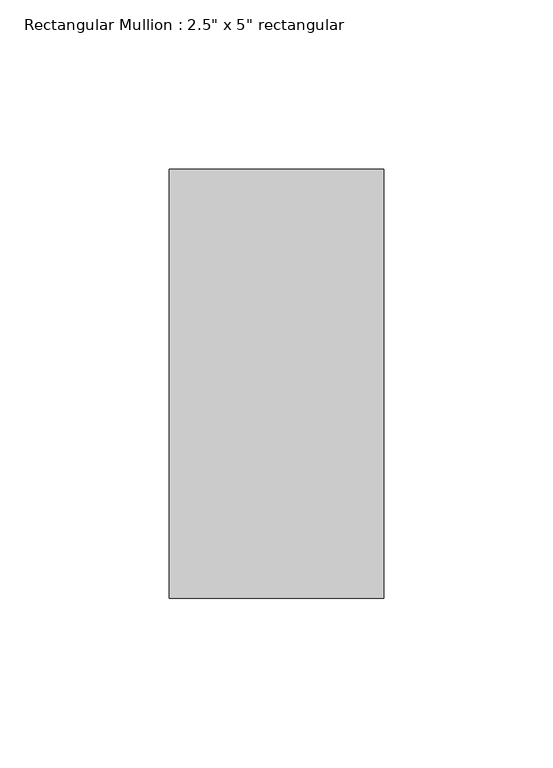
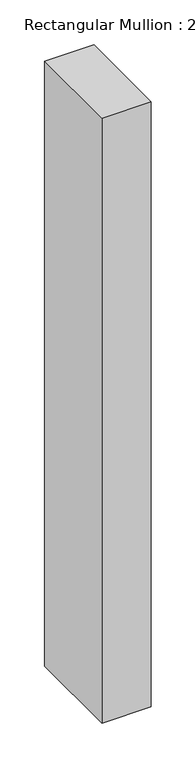
"""IFC4 building model written with IfcOpenShell, lengths in millimetres: member geometry."""

from ifc_helpers import new_model, si_unit, frame, origin, place, context, project, spatial, polyline, outline, extrude, source, transform, mapped, element, save


def member_eb0d2563(model_context):
    return source(origin(), model_context, "Body", "SweptSolid", [
        extrude(outline(polyline([(0.0, 63.5), (0.0, -63.5), (-63.5, -63.5), (-63.5, 63.5), (0.0, 63.5)])), frame((0.0, 0.0, -821.736197), z_axis=(0.0, 0.0, 1.0), x_axis=(1.0, 0.0, 0.0)), (0.0, 0.0, 1.0), 821.736197),
    ])


if __name__ == "__main__":
    model = new_model("IFC4")
    model_context = context("Model", 3, world=origin())
    ifc_project = project(units=[si_unit("LENGTHUNIT", "METRE", prefix="MILLI")], contexts=[model_context])
    site = spatial("IfcSite", under=ifc_project)
    building = spatial("IfcBuilding", under=site)
    placement = place(None, origin())
    member_shape = member_eb0d2563(model_context)
    element("IfcMember", 1, ObjectType="Rectangular Mullion : 2.5\" x 5\" rectangular", at=placement, inside=building, context=model_context, shape_type="MappedRepresentation", body=[
        mapped(member_shape, transform((0.0, 0.0, 0.0), x_axis=(1.0, 0.0, 0.0), y_axis=(0.0, 1.0, 0.0), z_axis=(0.0, 0.0, 1.0))),
    ])
    save(model, "model.ifc")

# Revit data of these elements
# Type "Rectangular Mullion : 2.5\" x 5\" rectangular"
#   built-in parameter 1007304 = 0.416667 (stored number, unit not read)
#   built-in parameter 1007301 = 0.104167 (stored number, unit not read)
#   built-in parameter 1007300 = 0.104167 (stored number, unit not read)
# Element 1 (IfcMember, "Rectangular Mullion : 2.5\" x 5\" rectangular")
#   Materials on its faces: "Aluminum"
# Materials
#   "Aluminum": class "Metal", colour RGB 247 247 247, transparency 0, Description = "Aluminum 6061", Cost = 0
